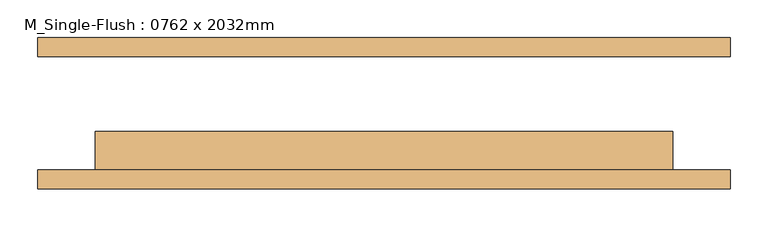
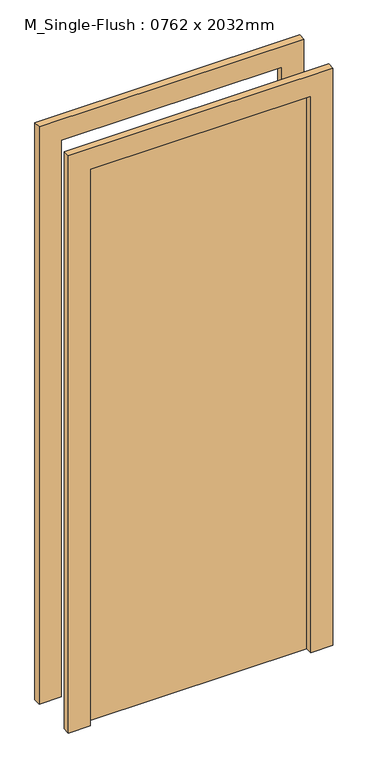
"""IFC4 building model written with IfcOpenShell, lengths in millimetres: door geometry, M_Single-Flush : 0762 x 2032mm."""

from ifc_helpers import new_model, si_unit, frame, origin, origin_with_axes, place, context, project, spatial, polyline, outline, extrude, source, transform, mapped, element, save


def m_single_flush_0762_x_2032mm_ffa3ef71(model_context):
    return source(origin(), model_context, "Body", "SweptSolid", [
        extrude(outline(polyline([(2108.0, -457.0), (0.0, -457.0), (0.0, -381.0), (2032.0, -381.0), (2032.0, 381.0), (0.0, 381.0), (0.0, 457.0), (2108.0, 457.0), (2108.0, -457.0)])), frame((0.0, -100.0, 0.0), z_axis=(0.0, 1.0, 0.0), x_axis=(0.0, 0.0, 1.0)), (0.0, 0.0, 1.0), 25.0),
        extrude(outline(polyline([(2108.0, 457.0), (2108.0, -457.0), (0.0, -457.0), (0.0, -381.0), (2032.0, -381.0), (2032.0, 381.0), (0.0, 381.0), (0.0, 457.0), (2108.0, 457.0)])), frame((0.0, 75.0, 0.0), z_axis=(0.0, 1.0, 0.0), x_axis=(0.0, 0.0, 1.0)), (0.0, 0.0, 1.0), 25.0),
        extrude(outline(polyline([(381.0, -24.0), (381.0, -75.0), (-381.0, -75.0), (-381.0, -24.0), (381.0, -24.0)])), origin_with_axes(), (0.0, 0.0, 1.0), 2032.0),
    ])


if __name__ == "__main__":
    model = new_model("IFC4")
    model_context = context("Model", 3, world=origin())
    ifc_project = project(units=[si_unit("LENGTHUNIT", "METRE", prefix="MILLI")], contexts=[model_context])
    site = spatial("IfcSite", under=ifc_project)
    building = spatial("IfcBuilding", under=site)
    placement = place(None, origin())
    m_single_flush_0762_x_2032mm_shape = m_single_flush_0762_x_2032mm_ffa3ef71(model_context)
    element("IfcDoor", 1, ObjectType="M_Single-Flush : 0762 x 2032mm", at=placement, inside=building, context=model_context, shape_type="MappedRepresentation", body=[
        mapped(m_single_flush_0762_x_2032mm_shape, transform((0.0, 0.0, 0.0), x_axis=(1.0, 0.0, 0.0), y_axis=(0.0, 1.0, 0.0), z_axis=(0.0, 0.0, 1.0))),
    ])
    save(model, "model.ifc")

# Revit data of these elements
# Type "M_Single-Flush : 0762 x 2032mm"
#   Type Mark = "19"
#   Thickness = 51 mm
#   Height = 2032 mm
#   Trim Projection Ext = 25 mm
#   Trim Projection Int = 25 mm
#   Trim Width = 76 mm
#   Width = 762 mm
#   Door Material = Door - Panel
#   Frame Material = Door - Frame
#   Function = (empty or 0)
#   Wall Closure = (empty or 0)
# Element 1 (IfcDoor, "M_Single-Flush : 0762 x 2032mm")
#   Materials on its faces: "Door - Frame", "Door - Panel"
# Materials
#   "Door - Panel": class "Wood", colour RGB 114 82 51, transparency 0
#   "Door - Frame": colour RGB 153 76 43, transparency 0
